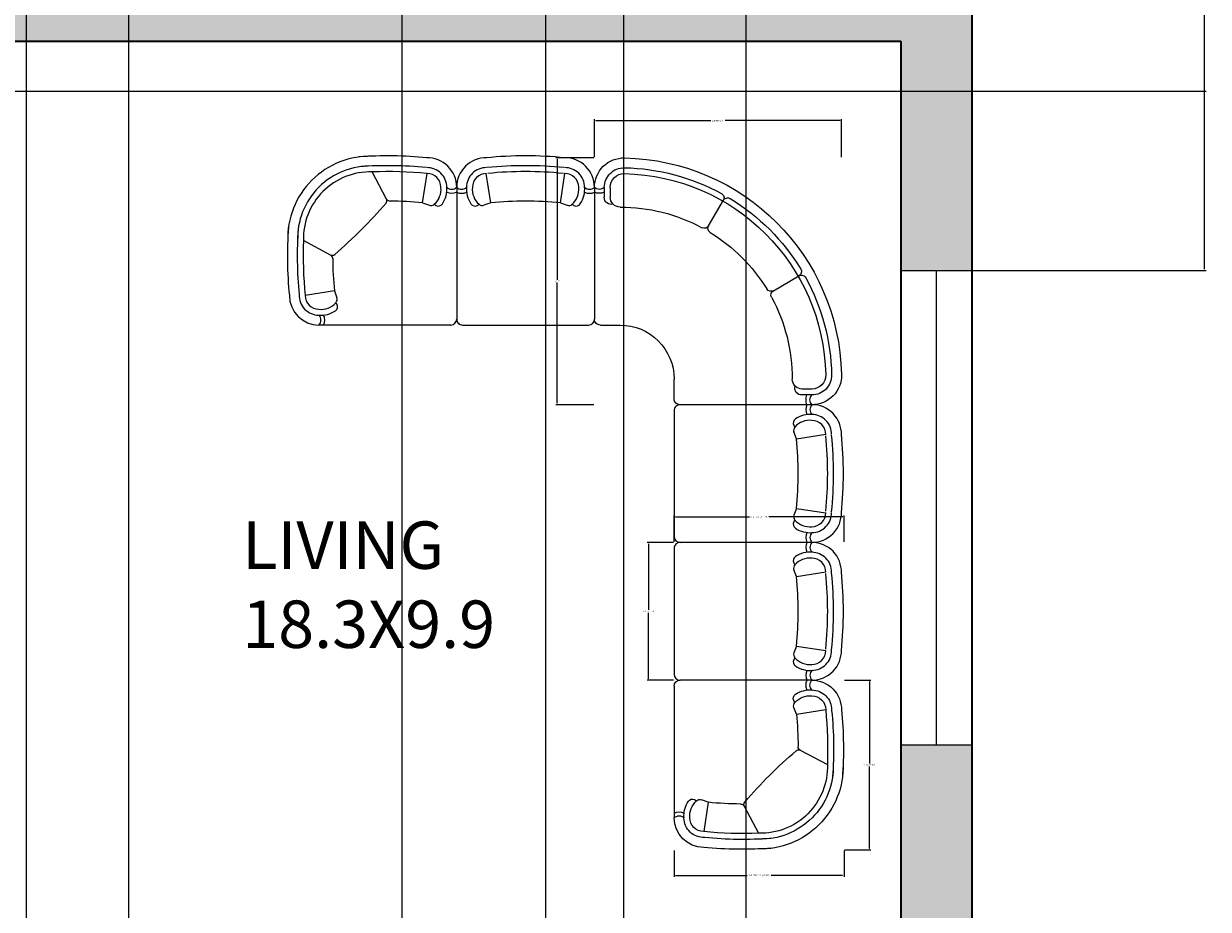
# Model space of a CAD drawing. Units: inches. Extents: x 0 to 423, y -517 to 94.
# Tile 4 of 8: x 273 to 423, y -382 to -270. Entities that reach past the tile are written whole.
import ezdxf

# ---------------------------------------------------------------- set-up
doc = ezdxf.new("R2010")
doc.units = ezdxf.units.IN
doc.header["$MEASUREMENT"] = 0
for name, color, linetype, lineweight in [('A-ANNO-DIMS', 2, 'Continuous', 18), ('A-AREA-IDEN', 7, 'Continuous', 18), ('A-FURN', 8, 'Continuous', 13), ('A-GLAZ', 4, 'Continuous', 18), ('A-WALL', 7, 'Continuous', 35)]:
    doc.layers.add(name, color=color, linetype=linetype, lineweight=lineweight)
doc.layers.add('A-WALL-PATT', color=30, linetype='Continuous', lineweight=13, true_color=0xf26722)
doc.styles.get("Standard").update_dxf_attribs({"font": 'arial.ttf'})
doc.dimstyles.get("Standard").update_dxf_attribs({"dimtxt": 0.18, "dimasz": 0.18, "dimexe": 0.18, "dimexo": 0.0625, "dimgap": 0.09, "dimtad": 0, "dimtih": 1, "dimtoh": 1, "dimdec": 0, "dimzin": 0, "dimdsep": 46, "dimlunit": 3, "dimtxsty": 'Standard', "dimcen": 0.09, "dimadec": 0, "dimazin": 0, "dimtfac": 1, "dimtdec": 0, "dimtofl": 0, "dimtmove": 0, "dimatfit": 3, "dimfxl": 1, "dimtolj": 1, "dimtzin": 0, "dimarcsym": 0})

# ---------------------------------------------------------------- blocks, each defined once
blk = doc.blocks.new('A$C707258B2')
at = {"color": 0}
for p, q in [((0.4042, 0.342), (1.0739, 0.342)), ((1.1039, 0.312), (1.1039, 0.212)), ((0.4042, 0.292), (0.4544, 0.292)), ((0.4042, 0.262), (0.4539, 0.262)), ((1.4789, -0.063), (1.3789, -0.063)), ((1.5089, -0.7628), (1.5089, -0.093)), ((0.5998, -0.2378), (0.4699, -0.3128)), ((0.9291, -0.5671), (0.8541, -0.697)), ((1.4289, -0.7628), (1.4289, -0.713)), ((1.4589, -0.7628), (1.4589, -0.7125))]:
    blk.add_line(p, q, dxfattribs=at)
for centre, radius, start, end in [((0.4042, 0.192), 0.15, 90, 181.17538), ((0.3779, 0.317), 0.0362, 316.39718, 43.60282), ((0.3679, 0.317), 0.0662, 337.82984, 22.17016), ((1.0739, 0.312), 0.03, 360, 90), ((0.4042, 0.192), 0.1, 90, 181.17538), ((0.4042, 0.192), 0.07, 90, 181.17538), ((0.4539, 0.212), 0.05, 360, 90), ((0.4548, 0.2564), 0.0357, 345.42616, 90.55549), ((1.3789, 0.212), 1.125, 181.17538, 268.82462), ((1.3789, 0.212), 1.075, 181.17538, 208.63569), ((1.3789, 0.212), 1.045, 181.17538, 268.82462), ((1.3789, 0.212), 0.875, 180, 208.40825), ((1.3789, 0.212), 0.275, 180, 270), ((1.4789, -0.093), 0.03, 360, 90), ((0.5873, -0.2162), 0.025, 300, 28.40825), ((0.6123, -0.2595), 0.025, 31.59175, 120), ((1.3789, 0.212), 0.875, 211.59175, 238.40825), ((0.4574, -0.2912), 0.025, 208.63569, 300), ((0.4824, -0.3345), 0.025, 120, 211.36431), ((1.3789, 0.212), 1.075, 211.36431, 238.63569), ((0.9075, -0.5546), 0.025, 330, 58.40825), ((0.9508, -0.5796), 0.025, 61.59175, 150), ((1.3789, 0.212), 0.875, 241.59175, 270), ((0.8324, -0.6845), 0.025, 238.63569, 330), ((0.8757, -0.7095), 0.025, 150, 241.36431), ((1.3789, -0.713), 0.05, 360, 90), ((1.4255, -0.7093), 0.0336, 354.63008, 109.38826), ((1.3789, 0.212), 1.075, 241.36431, 268.82462), ((1.3589, -0.7628), 0.15, 268.82462, 360), ((1.3589, -0.7628), 0.1, 268.82462, 360), ((1.3589, -0.7628), 0.07, 268.82462, 360), ((1.4839, -0.7988), 0.0662, 67.82984, 112.17016), ((1.4839, -0.789), 0.0362, 46.39718, 133.60282)]:
    blk.add_arc(centre, radius, start, end, dxfattribs=at)
blk = doc.blocks.new('part 01')
at = {"color": 0}
for p, q in [((-669.8, 700), (0, 700)), ((30, 30), (30, 670)), ((-590.9, 527.1), (-739.8, 550)), ((-590.9, 527.1), (-578.5, 561.2)), ((-590.9, 172.9), (-739.8, 150)), ((-590.9, 172.9), (-578.5, 138.8)), ((-669.8, 0), (0, 0))]:
    blk.add_line(p, q, dxfattribs=at)
for centre, radius, start, end in [((-669.8, 550), 150, 90, 181.17538), ((-696, 675), 36.2, 316.39718, 43.60282), ((-705.9, 675), 66.2, 337.82984, 22.17016), ((0, 670), 30, 0, 90), ((-669.8, 550), 100, 90, 181.17538), ((-669.8, 550), 70, 90, 181.17538), ((-659.7, 517.8), 132.7, 56.08973, 95.61316), ((-659.7, 517.8), 102.7, 42.00663, 95.61316), ((-599.7, 607.2), 25, 332.96082, 56.08973), ((1178.1, 350), 2007.9, 174.28354, 185.71646), ((1178.1, 350), 1957.9, 174.28354, 185.71646), ((1178.1, 350), 1927.9, 174.28354, 185.71646), ((-624.8, 620), 53.2, 321.00172, 332.96082), ((-602, 569.8), 25, 340, 42.00663), ((1178.1, 350), 1777.9, 174.28354, 185.71646), ((-669.8, 150), 150, 178.82462, 270), ((-669.8, 150), 100, 178.82462, 270), ((-669.8, 150), 70, 178.82462, 270), ((-602, 130.2), 25, 317.99337, 20), ((-659.7, 182.2), 132.7, 264.38684, 303.91027), ((-659.7, 182.2), 102.7, 264.38684, 317.99337), ((-599.7, 92.8), 25, 303.91027, 27.03918), ((-624.8, 80), 53.2, 27.03918, 38.99828), ((-696, 25), 36.2, 316.39718, 43.60282), ((-705.9, 25), 66.2, 337.82984, 22.17016), ((0, 30), 30, 270, 0)]:
    blk.add_arc(centre, radius, start, end, dxfattribs=at)
blk = doc.blocks.new('part02')
at = {"color": 0}
for p, q in [((0, -669.8), (0, 0)), ((30, 30), (699.8, 30)), ((620.9, -142.9), (608.5, -108.8)), ((620.9, -142.9), (769.8, -120)), ((640.4, -325.6), (778.2, -398.9)), ((172.9, -590.9), (138.8, -578.5)), ((172.9, -590.9), (150, -739.8)), ((355.6, -610.4), (428.9, -748.2))]:
    blk.add_line(p, q, dxfattribs=at)
for centre, radius, start, end in [((30, 0), 30, 90, 180), ((726, 5), 56.2, 153.6122, 206.66656), ((726, 5), 36.2, 136.39718, 223.60282), ((699.8, -120), 150, 0, 90), ((629.7, -62.8), 25, 123.91027, 207.03918), ((689.7, -152.2), 102.7, 84.38684, 137.99337), ((689.3, -151.3), 131.7, 85.43775, 123.98866), ((699.5, -120.6), 100.6, 357.50055, 89.85796), ((699.8, -120), 70, 0, 90), ((632, -100.2), 25, 137.99337, 200), ((654.8, -50), 53.2, 207.03918, 218.99828), ((-1228.2, -319.5), 2007.9, 357.73494, 5.70316), ((-1148.1, -320), 2007.9, 355.81801, 5.71646), ((-1148.1, -320), 1777.9, 0.38365, 5.71646), ((-1148.1, -320), 1957.9, 355.86566, 5.71646), ((2219.8, -2189.8), 2454.4, 130.6961, 139.3039), ((632.4, -344.1), 20, 62, 130.6961), ((649.7, -308), 20, 180.38365, 242), ((439.4, -409.4), 418.9, 268.21809, 1.78191), ((439.4, -409.4), 368.9, 268.21809, 1.78191), ((439.4, -409.4), 338.9, 268.21809, 1.78191), ((182.2, -659.7), 132.7, 146.08973, 185.61316), ((92.8, -599.7), 25, 62.96082, 146.08973), ((182.2, -659.7), 102.7, 132.00663, 185.61316), ((80, -624.8), 53.2, 51.00172, 62.96082), ((130.2, -602), 25, 70, 132.00663), ((350, 1178.1), 1777.9, 264.28354, 269.61635), ((338, -619.7), 20, 28, 89.61635), ((374.1, -602.4), 20, 139.3039, 208), ((25, -696), 56.2, 63.33344, 116.3878), ((25, -696), 36.2, 46.39718, 133.60282), ((150, -669.8), 150, 180, 271.17538), ((150, -669.8), 100, 180, 271.17538), ((150, -669.8), 70, 180, 270), ((349.5, 1258.2), 2007.9, 264.29684, 272.26506), ((350, 1178.1), 1957.9, 264.28354, 274.13434), ((350, 1178.1), 2007.9, 264.28354, 274.18199)]:
    blk.add_arc(centre, radius, start, end, dxfattribs=at)
blk = doc.blocks.new('WIN-GLAZ-60IN')
for p, q in [((0, 60), (0, 0)), ((4.5, 60), (4.5, 0)), ((9, 0), (9, 60))]:
    blk.add_line(p, q)
blk = doc.blocks.new('*D18')
at = {"layer": 'A-ANNO-DIMS', "color": 0, "lineweight": -2, "transparency": 16777216}
for p, q in [((355.09, -335.09), (355.09, -331.75)), ((355.27, -331.93), (364.61, -331.93)), ((376.38, -331.93), (367.03, -331.93)), ((376.56, -335.09), (376.56, -331.75))]:
    blk.add_line(p, q, dxfattribs=at)
at = {"layer": 'A-ANNO-DIMS', "color": 0, "transparency": 16777216}
for points in [[(355.27, -331.9), (355.27, -331.96), (355.09, -331.93)], [(376.38, -331.9), (376.38, -331.96), (376.56, -331.93)]]:
    blk.add_solid(points, dxfattribs=at)
at = {"layer": 'Defpoints', "color": 0, "transparency": 16777216}
for p in [(355.09, -331.93), (355.09, -335.15), (376.56, -335.15)]:
    blk.add_point(p, dxfattribs=at)
at = {"layer": 'A-ANNO-DIMS', "color": 0, "transparency": 16777216, "insert": (365.82, -331.93), "char_height": 0.18, "attachment_point": 5}
blk.add_mtext('\\A1;SEAT 1\'-9 1/2" TYP.', dxfattribs=at)
blk = doc.blocks.new('*D19')
at = {"layer": 'A-ANNO-DIMS', "color": 0, "lineweight": -2, "transparency": 16777216}
for p, q in [((355.02, -335.15), (351.68, -335.15)), ((351.86, -335.33), (351.86, -343.67)), ((351.86, -352.38), (351.86, -344.04)), ((355.02, -352.56), (351.68, -352.56))]:
    blk.add_line(p, q, dxfattribs=at)
at = {"layer": 'A-ANNO-DIMS', "color": 0, "transparency": 16777216}
for points in [[(351.83, -335.33), (351.89, -335.33), (351.86, -335.15)], [(351.83, -352.38), (351.89, -352.38), (351.86, -352.56)]]:
    blk.add_solid(points, dxfattribs=at)
at = {"layer": 'Defpoints', "color": 0, "transparency": 16777216}
for p in [(355.09, -335.15), (351.86, -352.56), (355.09, -352.56)]:
    blk.add_point(p, dxfattribs=at)
at = {"layer": 'A-ANNO-DIMS', "color": 0, "transparency": 16777216, "insert": (351.86, -343.86), "char_height": 0.18, "attachment_point": 5}
blk.add_mtext('\\A1;1\'-5 1/2" TYP.', dxfattribs=at)
blk = doc.blocks.new('*D20')
at = {"layer": 'A-ANNO-DIMS', "color": 0, "lineweight": -2, "transparency": 16777216}
for p, q in [((355.09, -374.09), (355.09, -377.43)), ((376.55, -374.09), (376.55, -377.43)), ((355.27, -377.25), (364.31, -377.25)), ((376.37, -377.25), (367.33, -377.25))]:
    blk.add_line(p, q, dxfattribs=at)
at = {"layer": 'A-ANNO-DIMS', "color": 0, "transparency": 16777216}
for points in [[(355.27, -377.22), (355.27, -377.28), (355.09, -377.25)], [(376.37, -377.22), (376.37, -377.28), (376.55, -377.25)]]:
    blk.add_solid(points, dxfattribs=at)
at = {"layer": 'Defpoints', "color": 0, "transparency": 16777216}
for p in [(355.09, -374.03), (376.55, -374.03), (355.09, -377.25)]:
    blk.add_point(p, dxfattribs=at)
at = {"layer": 'A-ANNO-DIMS', "color": 0, "transparency": 16777216, "insert": (365.82, -377.25), "char_height": 0.18, "attachment_point": 5}
blk.add_mtext('\\A1;END SEAT 1\'-9 1/2" TYP.', dxfattribs=at)
blk = doc.blocks.new('*D21')
at = {"layer": 'A-ANNO-DIMS', "color": 0, "lineweight": -2, "transparency": 16777216}
for p, q in [((376.61, -352.56), (379.95, -352.56)), ((379.77, -352.74), (379.77, -363.11)), ((379.77, -373.85), (379.77, -363.48)), ((376.61, -374.03), (379.95, -374.03))]:
    blk.add_line(p, q, dxfattribs=at)
at = {"layer": 'A-ANNO-DIMS', "color": 0, "transparency": 16777216}
for points in [[(379.74, -352.74), (379.8, -352.74), (379.77, -352.56)], [(379.74, -373.85), (379.8, -373.85), (379.77, -374.03)]]:
    blk.add_solid(points, dxfattribs=at)
at = {"layer": 'Defpoints', "color": 0, "transparency": 16777216}
for p in [(376.55, -352.56), (376.55, -374.03), (379.77, -374.03)]:
    blk.add_point(p, dxfattribs=at)
at = {"layer": 'A-ANNO-DIMS', "color": 0, "transparency": 16777216, "insert": (379.77, -363.3), "char_height": 0.18, "attachment_point": 5}
blk.add_mtext('\\A1;1\'-9 1/2" TYP.', dxfattribs=at)
blk = doc.blocks.new('*D22')
at = {"layer": 'A-ANNO-DIMS', "color": 0, "lineweight": -2, "transparency": 16777216}
for p, q in [((345.01, -286.44), (345.01, -281.63)), ((345.19, -281.81), (359.72, -281.81)), ((376.07, -281.81), (361.54, -281.81)), ((376.25, -286.44), (376.25, -281.63))]:
    blk.add_line(p, q, dxfattribs=at)
at = {"layer": 'A-ANNO-DIMS', "color": 0, "transparency": 16777216}
for points in [[(345.19, -281.78), (345.19, -281.84), (345.01, -281.81)], [(376.07, -281.78), (376.07, -281.84), (376.25, -281.81)]]:
    blk.add_solid(points, dxfattribs=at)
at = {"layer": 'Defpoints', "color": 0, "transparency": 16777216}
for p in [(345.01, -281.81), (345.01, -286.5), (376.25, -286.5)]:
    blk.add_point(p, dxfattribs=at)
at = {"layer": 'A-ANNO-DIMS', "color": 0, "transparency": 16777216, "insert": (360.63, -281.81), "char_height": 0.18, "attachment_point": 5}
blk.add_mtext('\\A1;CORNER 2\'-7"', dxfattribs=at)
blk = doc.blocks.new('*D23')
at = {"layer": 'A-ANNO-DIMS', "color": 0, "lineweight": -2, "transparency": 16777216}
for p, q in [((344.95, -286.5), (340.14, -286.5)), ((340.32, -286.68), (340.32, -301.94)), ((340.32, -317.55), (340.32, -302.3)), ((344.95, -317.73), (340.14, -317.73))]:
    blk.add_line(p, q, dxfattribs=at)
at = {"layer": 'A-ANNO-DIMS', "color": 0, "transparency": 16777216}
for points in [[(340.29, -286.68), (340.35, -286.68), (340.32, -286.5)], [(340.29, -317.55), (340.35, -317.55), (340.32, -317.73)]]:
    blk.add_solid(points, dxfattribs=at)
at = {"layer": 'Defpoints', "color": 0, "transparency": 16777216}
for p in [(345.01, -286.5), (340.32, -317.73), (345.01, -317.73)]:
    blk.add_point(p, dxfattribs=at)
at = {"layer": 'A-ANNO-DIMS', "color": 0, "transparency": 16777216, "insert": (340.32, -302.12), "char_height": 0.18, "attachment_point": 5}
blk.add_mtext('\\A1;2\'-7"', dxfattribs=at)
blk = doc.blocks.new('*D35')
at = {"layer": 'A-ANNO-DIMS', "color": 0, "lineweight": -2, "transparency": 16777216}
for p, q in [((320.72, -389.7), (320.72, 45.81)), ((320.9, 45.63), (334.39, 45.63)), ((348.54, 45.63), (335.05, 45.63)), ((348.72, -389.7), (348.72, 45.81))]:
    blk.add_line(p, q, dxfattribs=at)
at = {"layer": 'A-ANNO-DIMS', "color": 0, "transparency": 16777216}
for points in [[(320.9, 45.66), (320.9, 45.6), (320.72, 45.63)], [(348.54, 45.66), (348.54, 45.6), (348.72, 45.63)]]:
    blk.add_solid(points, dxfattribs=at)
at = {"layer": 'Defpoints', "color": 0, "transparency": 16777216}
for p in [(348.72, 45.63), (320.72, -389.77), (348.72, -389.77)]:
    blk.add_point(p, dxfattribs=at)
at = {"layer": 'A-ANNO-DIMS', "color": 0, "transparency": 16777216, "insert": (334.72, 45.63), "char_height": 0.18, "attachment_point": 5}
blk.add_mtext('\\A1;2\'-4"', dxfattribs=at)
blk = doc.blocks.new('*D44')
at = {"layer": 'A-ANNO-DIMS', "color": 0, "lineweight": -2, "transparency": 16777216}
for p, q in [((392.79, -229.77), (422.3, -229.77)), ((422.12, -229.95), (422.12, -265.08)), ((422.12, -300.59), (422.12, -265.45)), ((392.79, -300.77), (422.3, -300.77))]:
    blk.add_line(p, q, dxfattribs=at)
at = {"layer": 'A-ANNO-DIMS', "color": 0, "transparency": 16777216}
for points in [[(422.09, -229.95), (422.15, -229.95), (422.12, -229.77)], [(422.09, -300.59), (422.15, -300.59), (422.12, -300.77)]]:
    blk.add_solid(points, dxfattribs=at)
at = {"layer": 'Defpoints', "color": 0, "transparency": 16777216}
for p in [(392.72, -229.77), (392.72, -300.77), (422.12, -300.77)]:
    blk.add_point(p, dxfattribs=at)
at = {"layer": 'A-ANNO-DIMS', "color": 0, "transparency": 16777216, "insert": (422.12, -265.27), "char_height": 0.18, "attachment_point": 5}
blk.add_mtext('\\A1;5\'-11"', dxfattribs=at)
blk = doc.blocks.new('*D50')
at = {"layer": 'A-ANNO-DIMS', "color": 0, "lineweight": -2, "transparency": 16777216}
for p, q in [((273.19, -103.61), (273.19, -517.35)), ((364.14, -103.61), (364.14, -517.35)), ((273.37, -517.17), (318.34, -517.17)), ((363.96, -517.17), (318.99, -517.17))]:
    blk.add_line(p, q, dxfattribs=at)
at = {"layer": 'A-ANNO-DIMS', "color": 0, "transparency": 16777216}
for points in [[(273.37, -517.14), (273.37, -517.2), (273.19, -517.17)], [(363.96, -517.14), (363.96, -517.2), (364.14, -517.17)]]:
    blk.add_solid(points, dxfattribs=at)
at = {"layer": 'Defpoints', "color": 0, "transparency": 16777216}
for p in [(273.19, -103.55), (364.14, -103.55), (364.14, -517.17)]:
    blk.add_point(p, dxfattribs=at)
at = {"layer": 'A-ANNO-DIMS', "color": 0, "transparency": 16777216, "insert": (318.66, -517.17), "char_height": 0.18, "attachment_point": 5}
blk.add_mtext('\\A1;7\'-7"', dxfattribs=at)
blk = doc.blocks.new('*D51')
at = {"layer": 'A-ANNO-DIMS', "color": 0, "lineweight": -2, "transparency": 16777216}
for p, q in [((286.14, -253.61), (286.14, -517.35)), ((338.82, -253.61), (338.82, -517.35)), ((286.32, -517.17), (311.93, -517.17)), ((338.64, -517.17), (313.02, -517.17))]:
    blk.add_line(p, q, dxfattribs=at)
at = {"layer": 'A-ANNO-DIMS', "color": 0, "transparency": 16777216}
for points in [[(286.32, -517.14), (286.32, -517.2), (286.14, -517.17)], [(338.64, -517.14), (338.64, -517.2), (338.82, -517.17)]]:
    blk.add_solid(points, dxfattribs=at)
at = {"layer": 'Defpoints', "color": 0, "transparency": 16777216}
for p in [(286.14, -253.55), (338.82, -253.55), (338.82, -517.17)]:
    blk.add_point(p, dxfattribs=at)
at = {"layer": 'A-ANNO-DIMS', "color": 0, "transparency": 16777216, "insert": (312.48, -517.17), "char_height": 0.18, "attachment_point": 5}
blk.add_mtext('\\A1;4\'-4 1/2"', dxfattribs=at)
blk = doc.blocks.new('*D53')
at = {"layer": 'A-ANNO-DIMS', "color": 0, "lineweight": -2, "transparency": 16777216}
for p, q in [((85.83, -247.61), (422.3, -247.61)), ((422.12, -247.79), (422.12, -262.66)), ((422.12, -277.89), (422.12, -263.02)), ((80.68, -278.07), (422.3, -278.07))]:
    blk.add_line(p, q, dxfattribs=at)
at = {"layer": 'A-ANNO-DIMS', "color": 0, "transparency": 16777216}
for points in [[(422.09, -247.79), (422.15, -247.79), (422.12, -247.61)], [(422.09, -277.89), (422.15, -277.89), (422.12, -278.07)]]:
    blk.add_solid(points, dxfattribs=at)
at = {"layer": 'Defpoints', "color": 0, "transparency": 16777216}
for p in [(85.77, -247.61), (80.61, -278.07), (422.12, -278.07)]:
    blk.add_point(p, dxfattribs=at)
at = {"layer": 'A-ANNO-DIMS', "color": 0, "transparency": 16777216, "insert": (422.12, -262.84), "char_height": 0.18, "attachment_point": 5}
blk.add_mtext('\\A1;2\'-6 1/2"', dxfattribs=at)

msp = doc.modelspace()

# ---------------------------------------------------------------- hatches: boundary and pattern name
at = {"layer": 'A-WALL-PATT'}
h = msp.add_hatch(color=256, dxfattribs=at)
h.dxf.hatch_style = 1
h.paths.add_polyline_path([(201.52, 16.23), (138.22, 16.23), (138.22, 7.23), (177.72, 7.23), (177.72, -138.77), (186.72, -138.77), (186.72, -92.77), (251.72, -92.77), (251.72, -22.53), (242.72, -22.53), (242.72, -83.77), (186.72, -83.77), (186.72, 7.23), (201.52, 7.23)])
h.paths.add_polyline_path([(78.22, 16.23), (29.72, 16.23), (29.72, -31.27), (38.72, -31.27), (38.72, 7.23), (78.22, 7.23)])
h.paths.add_polyline_path([(275.31, 16.23), (225.52, 16.23), (225.52, 7.23), (275.31, 7.23)])
h.paths.add_polyline_path([(392.72, 16.23), (335.31, 16.23), (335.31, 7.23), (383.72, 7.23), (383.72, -31.27), (392.72, -31.27)])
h.paths.add_polyline_path([(143.33, -129.77), (38.72, -129.77), (38.72, -91.27), (29.72, -91.27), (29.72, -157.27), (38.72, -157.27), (38.72, -138.77), (143.33, -138.77)])
h.paths.add_polyline_path([(186.72, -199.77), (38.72, -199.77), (38.72, -181.27), (29.72, -181.27), (29.72, -239.27), (38.72, -239.27), (38.72, -208.77), (177.72, -208.77), (177.72, -237.07), (186.72, -237.07)])
h.paths.add_polyline_path([(111.72, -161.55), (102.72, -161.55), (102.72, -199.77), (111.72, -199.77)])
h.paths.add_polyline_path([(392.72, -91.27), (383.72, -91.27), (383.72, -129.77), (242.72, -129.77), (242.72, -138.77), (383.72, -138.77), (383.72, -169.77), (392.72, -169.77)])
h.paths.add_polyline_path([(392.72, -229.77), (383.72, -229.77), (383.72, -262.77), (251.72, -262.77), (251.72, -177.14), (242.72, -177.14), (242.72, -271.77), (383.72, -271.77), (383.72, -300.77), (392.72, -300.77)])
h.paths.add_polyline_path([(392.72, -360.77), (383.72, -360.77), (383.72, -389.77), (378.42, -389.77), (378.42, -398.77), (383.72, -398.77), (383.72, -458.77), (382.72, -458.77), (382.72, -467.77), (392.72, -467.77)])
h.paths.add_polyline_path([(364.92, -389.77), (348.72, -389.77), (348.72, -467.77), (358.72, -467.77), (358.72, -458.77), (357.72, -458.77), (357.72, -398.77), (364.92, -398.77)])
h.paths.add_polyline_path([(320.72, -389.77), (283.72, -389.77), (283.72, -398.77), (320.72, -398.77)])
h.paths.add_polyline_path([(223.72, -389.77), (186.72, -389.77), (186.72, -270.38), (177.72, -270.38), (177.72, -458.77), (138.22, -458.77), (138.22, -467.77), (186.72, -467.77), (186.72, -398.77), (223.72, -398.77)])
h.paths.add_polyline_path([(143.29, -329.77), (38.72, -329.77), (38.72, -299.27), (29.72, -299.27), (29.72, -338.77), (143.29, -338.77)])
h.paths.add_polyline_path([(38.72, -374.71), (29.72, -374.71), (29.72, -398.74), (38.72, -398.74)])
h.paths.add_polyline_path([(78.22, -458.77), (38.72, -458.77), (38.72, -434.74), (29.72, -434.74), (29.72, -467.77), (78.22, -467.77)])
h.paths.add_polyline_path([(279.99, -158.17), (326.6, -158.17), (326.6, -135.78), (279.99, -135.78)], flags=25)
h.paths.add_polyline_path([(355.56, -439.13), (387, -439.13), (387, -416.66), (355.56, -416.66)], flags=9)

# ---------------------------------------------------------------- linework, layer by layer
at = {"layer": 'A-GLAZ'}
for p, q in [((383.72, -300.77), (392.72, -300.77)), ((392.72, -360.77), (383.72, -360.77))]:
    msp.add_line(p, q, dxfattribs=at)
at = {"layer": 'A-WALL'}
for p, q in [((392.72, 16.23), (392.72, -467.77)), ((242.72, -271.77), (383.72, -271.77)), ((383.72, -271.77), (383.72, -389.77))]:
    msp.add_line(p, q, dxfattribs=at)

# ---------------------------------------------------------------- block references
at = {"layer": 'A-FURN', "ltscale": 0.03}
for name, p, xscale, yscale, zscale, rotation in [('part02', (327.6, -306.91), 0.0248775501551268, 0.0248775501551268, 0.0248775501551268, 180), ('part 01', (327.6, -306.91), 0.0248775501551268, 0.0248775501551268, 0.0248775501551268, 270), ('A$C707258B2', (353.52, -280.2), -24.87755015512683, 24.87755015512683, 24.87755015512683, 89.9999999999967), ('part 01', (355.83, -317.73), 0.0248775501551268, 0.0248775501551268, 0.0248775501551268, 180), ('part 01', (355.83, -335.15), 0.0248775501551268, 0.0248775501551268, 0.0248775501551268, 180), ('part02', (355.83, -352.56), -0.0248775501551268, 0.0248775501551268, 0.0248775501551268, 89.9999999999967)]:
    msp.add_blockref(name, p, dxfattribs=dict(at, xscale=xscale, yscale=yscale, zscale=zscale, rotation=rotation))
at = {"layer": 'A-GLAZ', "rotation": 180}
msp.add_blockref('WIN-GLAZ-60IN', (392.72, -300.77), dxfattribs=at)

# ---------------------------------------------------------------- texts
at = {"layer": 'A-AREA-IDEN', "insert": (300.5, -332.49), "char_height": 6, "attachment_point": 1}
msp.add_mtext('LIVING\\P18.3X9.9', dxfattribs=at)

# ---------------------------------------------------------------- dimensions: what is measured, and where the dimension line sits
at = {"layer": 'A-ANNO-DIMS'}
for base, p1, p2, picture, middle in [((348.72, 45.63), (320.72, -389.77), (348.72, -389.77), '*D35', (334.72, 45.63)), ((364.1422, -517.1651), (273.186, -103.5478), (364.1422, -103.5478), '*D50', (318.6641, -517.1651)), ((338.82, -517.17), (286.14, -253.55), (338.82, -253.55), '*D51', (312.48, -517.17))]:
    dim = msp.add_linear_dim(base=base, p1=p1, p2=p2, dimstyle='Standard', override={"dimdec": 1, "dimlfac": 1, "dimrnd": 0, "dimzin": 1, "dimdsep": 46, "dimlunit": 4, "dimfrac": 2}, dxfattribs=at)
    dim.commit()
    dim.dimension.update_dxf_attribs({"geometry": picture, "text_midpoint": middle})
for base, p1, p2, angle, picture, middle in [((422.12, -300.77), (392.72, -229.77), (392.72, -300.77), 270, '*D44', (422.12, -265.27)), ((422.12, -278.07), (85.77, -247.61), (80.61, -278.07), 90, '*D53', (422.12, -262.84)), ((340.32, -317.73), (345.01, -286.5), (345.01, -317.73), 270, '*D23', (340.32, -302.12))]:
    dim = msp.add_linear_dim(base=base, p1=p1, p2=p2, angle=angle, dimstyle='Standard', override={"dimdec": 1, "dimlfac": 1, "dimrnd": 0, "dimzin": 1, "dimdsep": 46, "dimlunit": 4, "dimfrac": 2}, dxfattribs=at)
    dim.commit()
    dim.dimension.update_dxf_attribs({"geometry": picture, "text_midpoint": middle})
for base, p1, p2, angle, text, picture, middle in [((345.01, -281.81), (376.25, -286.5), (345.01, -286.5), 180, 'CORNER <>', '*D22', (360.63, -281.81)), ((355.09, -331.93), (376.56, -335.15), (355.09, -335.15), 180, 'SEAT <> TYP.', '*D18', (365.82, -331.93)), ((351.86, -352.56), (355.09, -335.15), (355.09, -352.56), 270, '<> TYP.', '*D19', (351.86, -343.86)), ((379.77, -374.03), (376.55, -352.56), (376.55, -374.03), 270, '<> TYP.', '*D21', (379.77, -363.3)), ((355.09, -377.25), (376.55, -374.03), (355.09, -374.03), 180, 'END SEAT <> TYP.', '*D20', (365.82, -377.25))]:
    dim = msp.add_linear_dim(base=base, p1=p1, p2=p2, angle=angle, text=text, dimstyle='Standard', override={"dimdec": 1, "dimlfac": 1, "dimrnd": 0, "dimzin": 1, "dimdsep": 46, "dimlunit": 4, "dimfrac": 2}, dxfattribs=at)
    dim.commit()
    dim.dimension.update_dxf_attribs({"geometry": picture, "text_midpoint": middle})

doc.saveas('drawing.dxf')
